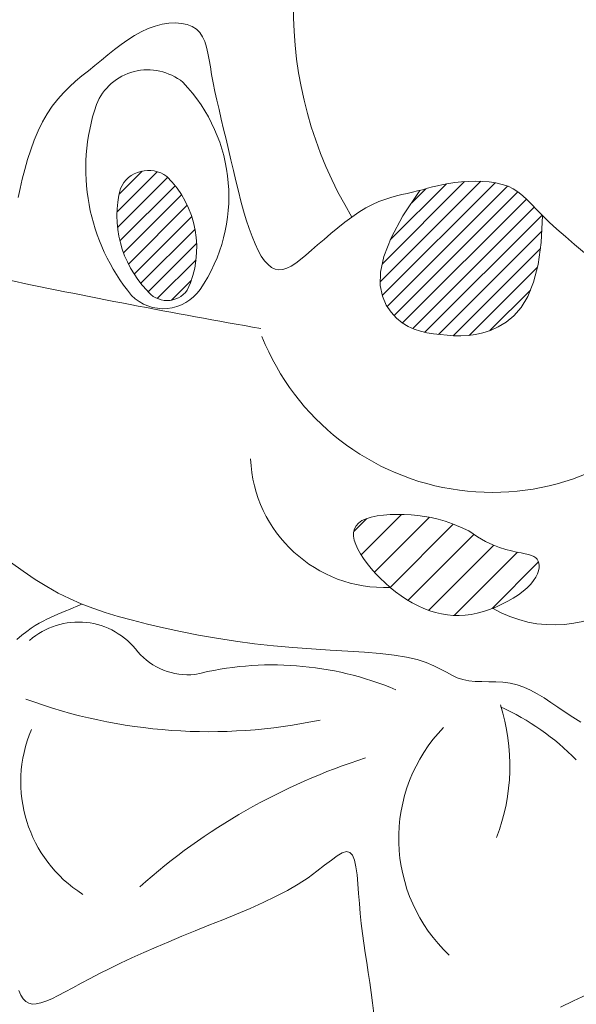
# Model space of a CAD drawing. Units: inches. Extents: x -17 to 1735, y -531 to 60.
# Tile 8 of 27: x 1734.673629 to 1734.675388, y -150.221388 to -150.218274. Entities that reach past the tile are written whole.
import ezdxf

# ---------------------------------------------------------------- set-up
doc = ezdxf.new("R2010")
doc.units = ezdxf.units.IN
doc.header["$MEASUREMENT"] = 0
doc.layers.add('A-FURN', color=242, linetype='Continuous', lineweight=18, true_color=0xcd2027)

# ---------------------------------------------------------------- blocks, each defined once
blk = doc.blocks.new('childrens_room_2')
for p, q in [((70.1409893039486, 54.10887213346581), (70.14043128957158, 54.10867226080739)), ((70.1415457864164, 54.10901436526041), (70.1409893039486, 54.10887213346581)), ((70.14209103538772, 54.10909844610291), (70.1415457864164, 54.10901436526041)), ((70.14261534933351, 54.10912386588319), (70.14209103538772, 54.10909844610291)), ((70.14310902649189, 54.10909011452026), (70.14261534933351, 54.10912386588319)), ((70.14356236527559, 54.10899668191126), (70.14310902649189, 54.10909011452026)), ((70.14396566403914, 54.10884305795338), (70.14356236527559, 54.10899668191126)), ((70.1443092211953, 54.10862873255831), (70.14396566403914, 54.10884305795338)), ((70.13933517482249, 54.10811183522895), (70.1387968190352, 54.1077663301316)), ((70.13987965789741, 54.10841653263054), (70.13933517482249, 54.10811183522895)), ((70.14043128957158, 54.10867226080739), (70.13987965789741, 54.10841653263054)), ((70.14458682429861, 54.10835379073836), (70.1443092211953, 54.10862873255831)), ((70.14480621752912, 54.10802069795903), (70.14458682429861, 54.10835379073836)), ((70.14497863449972, 54.10763251480097), (70.14480621752912, 54.10802069795903)), ((70.13826356939856, 54.10738817888199), (70.13773440460093, 54.10698554301638)), ((70.1387968190352, 54.1077663301316), (70.13826356939856, 54.10738817888199)), ((70.14511530859048, 54.10719230183753), (70.14497863449972, 54.10763251480097)), ((70.14522747323964, 54.10670311964935), (70.14511530859048, 54.10719230183753)), ((70.13720830350533, 54.106566584071), (70.13668424485834, 54.10613946358211)), ((70.13773440460093, 54.10698554301638), (70.13720830350533, 54.106566584071)), ((70.14532636200195, 54.10616802881708), (70.14522747323964, 54.10670311964935)), ((70.13616120746477, 54.10571234308594), (70.13563902106719, 54.1052905785968)), ((70.13668424485834, 54.10613946358211), (70.13616120746477, 54.10571234308594)), ((70.14542320831563, 54.10559008991407), (70.14532636200195, 54.10616802881708)), ((70.14552924561897, 54.10497236352097), (70.14542320831563, 54.10559008991407)), ((70.13512091956684, 54.10486830399753), (70.13461098786095, 54.10443684767819)), ((70.13563902106719, 54.1052905785968), (70.13512091956684, 54.10486830399753)), ((70.14565340960283, 54.10431791021841), (70.14552924561897, 54.10497236352097)), ((70.13411331084674, 54.10398753798512), (70.13363197342144, 54.10351170330108)), ((70.13461098786095, 54.10443684767819), (70.13411331084674, 54.10398753798512)), ((70.14579544502661, 54.10362979057248), (70.14565340960283, 54.10431791021841)), ((70.13363197342144, 54.10351170330108), (70.13317106054049, 54.10300067199426)), ((70.14595279878588, 54.10291106516382), (70.14579544502661, 54.10362979057248)), ((70.1327346569847, 54.1024457724256), (70.1323268477677, 54.10183833297054)), ((70.13317106054049, 54.10300067199426), (70.1327346569847, 54.1024457724256)), ((70.14612291789265, 54.10216479456579), (70.14595279878588, 54.10291106516382)), ((70.1323268477677, 54.10183833297054), (70.13195086667432, 54.10117316764666)), ((70.14630324918429, 54.10139403935176), (70.14612291789265, 54.10216479456579)), ((70.13195086667432, 54.10117316764666), (70.13160654356354, 54.1004590331126)), ((70.14649123967277, 54.10060186009508), (70.14630324918429, 54.10139403935176)), ((70.13160654356354, 54.1004590331126), (70.13129285718199, 54.09970817165453)), ((70.14668433631189, 54.09979131736912), (70.14649123967277, 54.10060186009508)), ((70.13129285718199, 54.09970817165453), (70.13100878633443, 54.09893282558044)), ((70.14687998593902, 54.09896547175453), (70.14668433631189, 54.09979131736912)), ((70.13100878633443, 54.09893282558044), (70.13075330982568, 54.09814523720564)), ((70.14707623132156, 54.09812823396936), (70.14687998593902, 54.09896547175453)), ((70.13075330982568, 54.09814523720564), (70.1305254063441, 54.09735764880901)), ((70.14727349795751, 54.09728691541244), (70.14707623132156, 54.09812823396936)), ((70.1305254063441, 54.09735764880901), (70.1303240547527, 54.09658230270583)), ((70.13792845654417, 54.09393505760675), (70.14116838924704, 54.09717499032416)), ((70.13809711784009, 54.09537651111026), (70.13995124435635, 54.09723063762652)), ((70.14747280698387, 54.09644967761273), (70.14727349795751, 54.09728691541244)), ((70.1303240547527, 54.09658230270583), (70.1301482338563, 54.09583144119682)), ((70.13797547931202, 54.09270928815243), (70.14199178125592, 54.09672559012546)), ((70.13816464070581, 54.09162565735318), (70.14259264316527, 54.09605365979809)), ((70.14767517977046, 54.09562468211373), (70.14747280698387, 54.09644967761273)), ((70.15907037753962, 54.08834834226439), (70.16712777678507, 54.09640574153167)), ((70.1592271576624, 54.0872323302014), (70.16828360648243, 54.09628877902145)), ((70.15923180711573, 54.08978256406266), (70.16583344911808, 54.09638420604318)), ((70.15987140628161, 54.09169495545069), (70.16437979241485, 54.09620334157665)), ((70.16366790474743, 54.09605469296224), (70.16325226613438, 54.09595114353436)), ((70.164101925398, 54.096151101045), (70.16366790474743, 54.09605469296224)), ((70.16456045543192, 54.09623730720927), (70.164101925398, 54.096151101045)), ((70.16504962225329, 54.09631025088896), (70.16456045543192, 54.09623730720927)), ((70.16557265970508, 54.09636678649116), (70.16504962225329, 54.09631025088896)), ((70.16612122779362, 54.09640342835195), (70.16557265970508, 54.09636678649116)), ((70.16668409296427, 54.09641660580968), (70.16612122779362, 54.09640342835195)), ((70.16725002189517, 54.0964027481736), (70.16668409296427, 54.09641660580968)), ((70.16780778097339, 54.09635828478934), (70.16725002189517, 54.0964027481736)), ((70.16834613681888, 54.09627964495888), (70.16780778097339, 54.09635828478934)), ((70.16885385587696, 54.09616325802057), (70.16834613681888, 54.09627964495888)), ((70.16931970470935, 54.09600555330547), (70.16885385587696, 54.09616325802057)), ((70.1301482338563, 54.09583144119682), (70.12999662443647, 54.09511539372619)), ((70.1384615440725, 54.09064976854137), (70.14312020183891, 54.09530842628595)), ((70.14788163739607, 54.09482009045899), (70.14767517977046, 54.09562468211373)), ((70.15962358274149, 54.08635596305106), (70.16928494146444, 54.09601732177401)), ((70.16017334769597, 54.08563293579795), (70.17010568234721, 54.09556527044191)), ((70.16080813407783, 54.09533562778818), (70.16036577337539, 54.09523063297678)), ((70.16123619758174, 54.0954314408504), (70.16080813407783, 54.09533562778818)), ((70.16088463407824, 54.09363122643703), (70.16225299740793, 54.09568155790333)), ((70.16165098525701, 54.09552674379523), (70.16123619758174, 54.0954314408504)), ((70.16158640251845, 54.09468274388058), (70.16270888149623, 54.09580522286564)), ((70.16205436912017, 54.0956282528918), (70.16165098525701, 54.09552674379523)), ((70.1624516256957, 54.09573486292214), (70.16205436912017, 54.0956282528918)), ((70.16284888227122, 54.09584351332745), (70.1624516256957, 54.09573486292214)), ((70.16325226613438, 54.09595114353436), (70.16284888227122, 54.09584351332745)), ((70.1697372155136, 54.09580355523798), (70.16931970470935, 54.09600555330547)), ((70.17011898343802, 54.09555666871023), (70.1697372155136, 54.09580355523798)), ((70.1704823693249, 54.09526489372223), (70.17011898343802, 54.09555666871023)), ((70.17084473395838, 54.09492823028125), (70.1704823693249, 54.09526489372223)), ((70.13884727908183, 54.08976271130672), (70.14356995939627, 54.09448539164299)), ((70.14809320123052, 54.09404406418474), (70.14788163739607, 54.09482009045899)), ((70.15843293467654, 54.09454540371228), (70.15790376987891, 54.09426442574335)), ((70.15894269618323, 54.09477384179485), (70.15843293467654, 54.09454540371228)), ((70.1594340756524, 54.09495841160827), (70.15894269618323, 54.09477384179485)), ((70.15990809433745, 54.09510778479893), (70.1594340756524, 54.09495841160827)), ((70.16036577337539, 54.09523063297678), (70.15990809433745, 54.09510778479893)), ((70.16084164999077, 54.08502844591424), (70.17079118512223, 54.09497798106753)), ((70.17122343823895, 54.09454667837275), (70.17084473395838, 54.09492823028125)), ((70.17163584289258, 54.09412023801127), (70.17122343823895, 54.09454667837275)), ((70.14831089235261, 54.09330476484178), (70.14809320123052, 54.09404406418474)), ((70.15735554230515, 54.09392572190558), (70.15679403878633, 54.09353804885762)), ((70.15790376987891, 54.09426442574335), (70.15735554230515, 54.09392572190558)), ((70.1616657237278, 54.08457972743639), (70.17142463272786, 54.09433863645102)), ((70.1626409005362, 54.08428211201538), (70.17205388856704, 54.09369510007531)), ((70.17209930887796, 54.09364890918226), (70.17163584289258, 54.09412023801127)), ((70.1393106744031, 54.08895331444949), (70.14393328998588, 54.09357593001772)), ((70.14853573207395, 54.09261035395906), (70.14831089235261, 54.09330476484178)), ((70.15622640797984, 54.09311364889294), (70.15565979836859, 54.09266476431952)), ((70.15679403878633, 54.09353804885762), (70.15622640797984, 54.09311364889294)), ((70.1599383932294, 54.09186810651448), (70.16088463407824, 54.09363122643703)), ((70.17209930887796, 54.09364890918226), (70.1719896525133, 54.09150446250572)), ((70.17263119697921, 54.09313269190755), (70.17209930887796, 54.09364890918226)), ((70.17324350653101, 54.09257243632459), (70.17263119697921, 54.09313269190755)), ((70.13984510513139, 54.08821495293381), (70.14419506136213, 54.09256490920819)), ((70.14876857144876, 54.09196839797226), (70.14853573207395, 54.09261035395906)), ((70.15510135855178, 54.09220363744537), (70.15455823712867, 54.09174251057123)), ((70.15565979836859, 54.09266476431952), (70.15510135855178, 54.09220363744537)), ((70.16374023003621, 54.08410864933689), (70.17203565414414, 54.09240407345208)), ((70.1739267913031, 54.09197239324424), (70.17324350653101, 54.09257243632459)), ((70.14043469169295, 54.08753174733141), (70.14432797663497, 54.09142503227343)), ((70.14900958061801, 54.09138408285656), (70.14876857144876, 54.09196839797226)), ((70.14925875963993, 54.09086199947927), (70.14900958061801, 54.09138408285656)), ((70.15403758264031, 54.09129362599782), (70.15354654368596, 54.09086922604041)), ((70.15455823712867, 54.09174251057123), (70.15403758264031, 54.09129362599782)), ((70.1593574794347, 54.0903665324426), (70.1599383932294, 54.09186810651448)), ((70.1719896525133, 54.09150446250572), (70.17173998460524, 54.08973568610822)), ((70.17466624338297, 54.09133766362941), (70.1739267913031, 54.09197239324424)), ((70.17544705514914, 54.09067334845025), (70.17466624338297, 54.09133766362941)), ((70.1495161083981, 54.09040673870044), (70.14925875963993, 54.09086199947927)), ((70.15354654368596, 54.09086922604041), (70.15309048165685, 54.09048061781362)), ((70.16490909830785, 54.08400472543002), (70.1719207591482, 54.09101638622672)), ((70.14116719552433, 54.08699145893336), (70.14427654911881, 54.09010081250603)), ((70.14978162700893, 54.0900228913801), (70.1495161083981, 54.09040673870044)), ((70.15005531541422, 54.08971504838558), (70.14978162700893, 54.0900228913801)), ((70.15033717361396, 54.08948780058421), (70.15005531541422, 54.08971504838558)), ((70.15227435268346, 54.08984010710122), (70.15190713713994, 54.08960146711473)), ((70.15266760940315, 54.09013536774586), (70.15227435268346, 54.08984010710122)), ((70.15309048165685, 54.09048061781362), (70.15266760940315, 54.09013536774586)), ((70.15908509709291, 54.08910083852828), (70.1593574794347, 54.0903665324426)), ((70.17173998460524, 54.08973568610822), (70.17137219559984, 54.08830158180939)), ((70.15062720160816, 54.08934573883602), (70.15033717361396, 54.08948780058421)), ((70.15092599509401, 54.08929158365066), (70.15062720160816, 54.08934573883602)), ((70.15123653267393, 54.08932057414353), (70.15092599509401, 54.08929158365066)), ((70.15156238858938, 54.08942607904322), (70.15123653267393, 54.08932057414353)), ((70.15190713713994, 54.08960146711473), (70.15156238858938, 54.08942607904322)), ((70.1590644508938, 54.08804535909297), (70.15908509709291, 54.08910083852828)), ((70.16620839743294, 54.08403123232568), (70.17168036016986, 54.08950319506988)), ((70.14231109433925, 54.08686256552613), (70.14389058733244, 54.08844205856297)), ((70.17137219559984, 54.08830158180939), (70.1709081759432, 54.08716115143619)), ((70.15923874523608, 54.0871744284363), (70.1590644508938, 54.08804535909297)), ((70.16787284421619, 54.08442288687223), (70.17111196486395, 54.08766200757094)), ((70.15955118469313, 54.08646238087243), (70.15923874523608, 54.0871744284363)), ((70.1709081759432, 54.08716115143619), (70.17036981608138, 54.08627339679373)), ((70.15994497378009, 54.08588355070827), (70.15955118469313, 54.08646238087243)), ((70.16037242878113, 54.08541446645398), (70.15994497378009, 54.08588355070827)), ((70.17036981608138, 54.08627339679373), (70.16977900640225, 54.08559731971621)), ((70.16082231311478, 54.08504043337456), (70.16037242878113, 54.08541446645398)), ((70.16129250179395, 54.08474895096009), (70.16082231311478, 54.08504043337456)), ((70.1691576372937, 54.08509192200148), (70.1685275993182, 54.08471620548374)), ((70.16977900640225, 54.08559731971621), (70.1691576372937, 54.08509192200148)), ((70.1617808700062, 54.08452751865701), (70.16129250179395, 54.08474895096009)), ((70.16228529288085, 54.08436363595541), (70.1617808700062, 54.08452751865701)), ((70.16280364548903, 54.08424480231627), (70.16228529288085, 54.08436363595541)), ((70.16333380296012, 54.08415851721514), (70.16280364548903, 54.08424480231627)), ((70.16729894659832, 54.08423096492919), (70.16670268169722, 54.08409601430907)), ((70.1679070163623, 54.08443431467316), (70.16729894659832, 54.08423096492919)), ((70.1685275993182, 54.08471620548374), (70.1679070163623, 54.08443431467316)), ((70.16387364048163, 54.084092280113), (70.16333380296012, 54.08415851721514)), ((70.16442150530521, 54.08403736424083), (70.16387364048163, 54.084092280113)), ((70.1649776335212, 54.08400013777868), (70.16442150530521, 54.08403736424083)), ((70.16554273351679, 54.0839907426693), (70.1649776335212, 54.08400013777868)), ((70.16611751344638, 54.08401932087002), (70.16554273351679, 54.0839907426693)), ((70.16670268169722, 54.08409601430907), (70.16611751344638, 54.08401932087002)), ((70.15694353497705, 54.06828989399077), (70.15797352163239, 54.06931988068248)), ((70.15731488378836, 54.06896104964693), (70.15758673929261, 54.06915109147525)), ((70.15752426960854, 54.06640090262084), (70.16076704901528, 54.069643682013)), ((70.15758673929261, 54.06915109147525), (70.15793346800959, 54.06930778243844)), ((70.15793346800959, 54.06930778243844), (70.15834586818121, 54.06943234820068)), ((70.15834586818121, 54.06943234820068), (70.15881212289563, 54.06952672402116)), ((70.15859754279839, 54.06500444983834), (70.1630163224286, 54.06942322947583)), ((70.15881212289563, 54.06952672402116), (70.15932041512454, 54.06959284515181)), ((70.15932041512454, 54.06959284515181), (70.15985892789789, 54.06963264684458)), ((70.15985892789789, 54.06963264684458), (70.16041584418738, 54.06964806436594)), ((70.16041584418738, 54.06964806436594), (70.16097934708117, 54.06964103295326)), ((70.16097934708117, 54.06964103295326), (70.16153761943454, 54.06961348786575)), ((70.16153761943454, 54.06961348786575), (70.16208233144019, 54.06956626772302)), ((70.16208233144019, 54.06956626772302), (70.16261910083588, 54.06949582454257)), ((70.16261910083588, 54.06949582454257), (70.16315703252215, 54.06939751371687)), ((70.16315703252215, 54.06939751371687), (70.16370523145773, 54.06926669061653)), ((70.16370523145773, 54.06926669061653), (70.16427280242672, 54.06909871063402)), ((70.15692550416455, 54.06820978447507), (70.15698814067176, 54.06848807385398)), ((70.15698814067176, 54.06848807385398), (70.15711664246513, 54.06873926967676)), ((70.15711664246513, 54.06873926967676), (70.15731488378836, 54.06896104964693)), ((70.15985669091927, 54.06379387196506), (70.16492787831115, 54.06886505934966)), ((70.16427280242672, 54.06909871063402), (70.16486885027146, 54.06888892915453)), ((70.16486885027146, 54.06888892915453), (70.16550247995067, 54.06863270154866)), ((70.16550247995067, 54.06863270154866), (70.16618279630669, 54.06832538321618)), ((70.15692485846697, 54.06790672385835), (70.15692550416455, 54.06820978447507)), ((70.15698232910248, 54.06758121430033), (70.15692485846697, 54.06790672385835)), ((70.15709404165275, 54.06723557809749), (70.15698232910248, 54.06758121430033)), ((70.16129145702465, 54.06275891204717), (70.16658396752203, 54.06805142253)), ((70.16618279630669, 54.06832538321618), (70.16686627735501, 54.06785863249973)), ((70.16686627735501, 54.06785863249973), (70.16750345904032, 54.06748961203851)), ((70.15725612175768, 54.06687213756089), (70.15709404165275, 54.06723557809749)), ((70.15746463044663, 54.06649356977727), (70.15725612175768, 54.06687213756089)), ((70.16295105697237, 54.06194878599348), (70.16817510856664, 54.06717283760958)), ((70.16750345904032, 54.06748961203851), (70.16809453501949, 54.06720458154308)), ((70.16809453501949, 54.06720458154308), (70.16863969906584, 54.06698980071673)), ((70.16863969906584, 54.06698980071673), (70.16913914489444, 54.06683152927001)), ((70.16913914489444, 54.06683152927001), (70.16959306616221, 54.06671602689897)), ((70.15771537030699, 54.06610397104526), (70.15746463044663, 54.06649356977727)), ((70.15800407949021, 54.06570779243924), (70.15771537030699, 54.06610397104526)), ((70.16500926205075, 54.06153726508495), (70.1700851896999, 54.06661319274866)), ((70.16959306616221, 54.06671602689897), (70.17000165670063, 54.06662955331416)), ((70.17000165670063, 54.06662955331416), (70.17036511016661, 54.06655836822614)), ((70.17036511016661, 54.06655836822614), (70.17068387854263, 54.06649040855558)), ((70.17068387854263, 54.06649040855558), (70.17095944711357, 54.06642032009989)), ((70.17095944711357, 54.06642032009989), (70.1711935593153, 54.06634442588842)), ((70.1711935593153, 54.06634442588842), (70.17138795870008, 54.06625904893593)), ((70.17138795870008, 54.06625904893593), (70.17154438864557, 54.06616051225722)), ((70.17154438864557, 54.06616051225722), (70.17166459270405, 54.06604513887436)), ((70.17166459270405, 54.06604513887436), (70.17175031442778, 54.06590925180939)), ((70.12938824494952, 54.06582249374918), (70.13038629923133, 54.06508380538292)), ((70.15832649626421, 54.06530948504808), (70.15800407949021, 54.06570779243924)), ((70.15867835860584, 54.06491349994616), (70.15832649626421, 54.06530948504808)), ((70.1680364764866, 54.06209475351937), (70.17177534610849, 54.06583362314126)), ((70.17175031442778, 54.06590925180939), (70.17180329719443, 54.06574917408438)), ((70.17181182089146, 54.06535128597756), (70.17176232505474, 54.06511924909722)), ((70.17180329719443, 54.06574917408438), (70.17182450963767, 54.06556242212395)), ((70.17182450963767, 54.06556242212395), (70.17181182089146, 54.06535128597756)), ((70.13038629923133, 54.06508380538292), (70.13135836332688, 54.06442877838566)), ((70.13135836332688, 54.06442877838566), (70.13229673647905, 54.06385020058809)), ((70.1590554047248, 54.06452428822234), (70.15867835860584, 54.06491349994616)), ((70.15945337271435, 54.06414630095827), (70.1590554047248, 54.06452428822234)), ((70.17154128902942, 54.06460640696463), (70.17136393715512, 54.06433256862368)), ((70.17167311640108, 54.06486979494224), (70.17154128902942, 54.06460640696463)), ((70.17176232505474, 54.06511924909722), (70.17167311640108, 54.06486979494224)), ((70.13229673647905, 54.06385020058809), (70.13321296988173, 54.06333893653794)), ((70.15986800066779, 54.06378398922829), (70.15945337271435, 54.06414630095827)), ((70.16029547889369, 54.06344138482968), (70.15986800066779, 54.06378398922829)), ((70.17086103670184, 54.06376747465987), (70.17053141993122, 54.06348331496559)), ((70.17113815499354, 54.06405176337142), (70.17086103670184, 54.06376747465987)), ((70.17136393715512, 54.06433256862368), (70.17113815499354, 54.06405176337142)), ((70.13321296988173, 54.06333893653794), (70.13412342757104, 54.06288536999494)), ((70.13412342757104, 54.06288536999494), (70.13504447393237, 54.06247988471881)), ((70.16073380545598, 54.0631208422987), (70.16029547889369, 54.06344138482968)), ((70.16118143063389, 54.0628242969164), (70.16073380545598, 54.0631208422987)), ((70.16163680464845, 54.06255368392016), (70.16118143063389, 54.0628242969164)), ((70.16973968119012, 54.06293202581441), (70.16929266934633, 54.06267341146161)), ((70.1701551164256, 54.06320341283429), (70.16973968119012, 54.06293202581441)), ((70.17053141993122, 54.06348331496559), (70.1701551164256, 54.06320341283429)), ((70.13381352038007, 54.06189630216835), (70.13412075077534, 54.06202414168223)), ((70.13412075077534, 54.06202414168223), (70.13440788049368, 54.06214337407295)), ((70.13440788049368, 54.06214337407295), (70.13466391713476, 54.06224951902408)), ((70.13466391713476, 54.06224951902408), (70.13487786853104, 54.06233809618282)), ((70.13487786853104, 54.06233809618282), (70.13503874234041, 54.06240462523277)), ((70.13503874234041, 54.06240462523277), (70.1351355462789, 54.06244462582112)), ((70.13504447393237, 54.06247988471881), (70.13599247300183, 54.06211286444744)), ((70.13599247300183, 54.06211286444744), (70.1369837890484, 54.06177469293329)), ((70.1620983777789, 54.06231093857645), (70.16163680464845, 54.06255368392016)), ((70.16256460024627, 54.06209799614448), (70.1620983777789, 54.06231093857645)), ((70.16303392227158, 54.06191679187617), (70.16256460024627, 54.06209799614448)), ((70.16833413655289, 54.06221153099472), (70.16783772578813, 54.06201677999201)), ((70.168821636074, 54.06243182733163), (70.16833413655289, 54.06221153099472)), ((70.16929266934633, 54.06267341146161), (70.168821636074, 54.06243182733163)), ((70.13199226559257, 54.06108987538613), (70.1322883098724, 54.06123859779331)), ((70.1322883098724, 54.06123859779331), (70.13258202177124, 54.06137478726162)), ((70.13258202177124, 54.06137478726162), (70.13287847088534, 54.06150423272487)), ((70.13287847088534, 54.06150423272487), (70.1331827266363, 54.06163272313136)), ((70.1331827266363, 54.06163272313136), (70.13349718159182, 54.06176433587683)), ((70.13349718159182, 54.06176433587683), (70.13381352038007, 54.06189630216835)), ((70.1369837890484, 54.06177469293329), (70.13803478622461, 54.06145575393606)), ((70.13803478622461, 54.06145575393606), (70.13916182874121, 54.06114643120822)), ((70.16350479407586, 54.06176926102347), (70.16303392227158, 54.06191679187617)), ((70.16397605336854, 54.06165698405533), (70.16350479407586, 54.06176926102347)), ((70.1644480875216, 54.06158012223608), (70.16397605336854, 54.06165698405533)), ((70.16492167151183, 54.06153848203979), (70.1644480875216, 54.06158012223608)), ((70.16539758014144, 54.06153186993328), (70.16492167151183, 54.06153848203979)), ((70.16587658832898, 54.06156009239061), (70.16539758014144, 54.06153186993328)), ((70.16635947093485, 54.06162295589314), (70.16587658832898, 54.06156009239061)), ((70.16684700287763, 54.06172026690041), (70.16635947093485, 54.06162295589314)), ((70.1673399589595, 54.06185183188648), (70.16684700287763, 54.06172026690041)), ((70.16783772578813, 54.06201677999201), (70.1673399589595, 54.06185183188648)), ((70.13068337576581, 54.0602538774678), (70.13103944413481, 54.0605106210773)), ((70.13103944413481, 54.0605106210773), (70.1313729022618, 54.06073167596918)), ((70.1313729022618, 54.06073167596918), (70.13168881956838, 54.06092283109177)), ((70.13168881956838, 54.06092283109177), (70.13199226559257, 54.06108987538613)), ((70.13916182874121, 54.06114643120822), (70.14037662821241, 54.06083951255863)), ((70.14037662821241, 54.06083951255863), (70.14167228598265, 54.06053740204374)), ((70.14167228598265, 54.06053740204374), (70.14303725091625, 54.06024490779822)), ((70.12990142278025, 54.05961865505236), (70.13030191418832, 54.0599567170488)), ((70.13030191418832, 54.0599567170488), (70.13068337576581, 54.0602538774678)), ((70.14303725091625, 54.06024490779822), (70.1444599717611, 54.05996683792768)), ((70.1444599717611, 54.05996683792768), (70.14592889732333, 54.05970800055951)), ((70.14592889732333, 54.05970800055951), (70.14743247646723, 54.05947320382842)), ((70.14743247646723, 54.05947320382842), (70.1489591579407, 54.05926725583999)), ((70.1489591579407, 54.05926725583999), (70.15049739060808, 54.05909496472162)), ((70.15049739060808, 54.05909496472162), (70.15203433979653, 54.05895857426952)), ((70.15203433979653, 54.05895857426952), (70.15355203697575, 54.05885007092587)), ((70.15355203697575, 54.05885007092587), (70.15503123013653, 54.05875887683072)), ((70.15503123013653, 54.05875887683072), (70.15645266744426, 54.05867441410231)), ((70.15645266744426, 54.05867441410231), (70.1577970967733, 54.05858610486615)), ((70.1577970967733, 54.05858610486615), (70.15904526628904, 54.05848337124047)), ((70.15904526628904, 54.05848337124047), (70.16017792398227, 54.05835563535077)), ((70.16017792398227, 54.05835563535077), (70.16117581784377, 54.05819231932986)), ((70.16117581784377, 54.05819231932986), (70.1620269154769, 54.05798685207122)), ((70.1620269154769, 54.05798685207122), (70.16274806223694, 54.05774868954762)), ((70.16274806223694, 54.05774868954762), (70.16336332320817, 54.05749129452164)), ((70.16336332320817, 54.05749129452164), (70.1638967632421, 54.0572281297413)), ((70.1638967632421, 54.0572281297413), (70.16437244742295, 54.0569726579692)), ((70.16437244742295, 54.0569726579692), (70.164814440544, 54.05673834194607)), ((70.164814440544, 54.05673834194607), (70.16524680774776, 54.05653864443451)), ((70.16524680774776, 54.05653864443451), (70.16569361388568, 54.05638702818254)), ((70.16569361388568, 54.05638702818254), (70.16617379006814, 54.05629198755781)), ((70.16617379006814, 54.05629198755781), (70.1666857319756, 54.05624214331914)), ((70.1666857319756, 54.05624214331914), (70.16722270148924, 54.05622114783767)), ((70.16722270148924, 54.05622114783767), (70.16777796031559, 54.05621265349186)), ((70.16777796031559, 54.05621265349186), (70.16834477033584, 54.0562003126601)), ((70.16834477033584, 54.0562003126601), (70.16891639337294, 54.05616777770632)), ((70.16891639337294, 54.05616777770632), (70.16948609124987, 54.05609870100164)), ((70.16948609124987, 54.05609870100164), (70.17004712567316, 54.05597673492451)), ((70.17004712567316, 54.05597673492451), (70.17059491488502, 54.05578987813209)), ((70.17059491488502, 54.05578987813209), (70.17113350216415, 54.05554351444738)), ((70.17113350216415, 54.05554351444738), (70.17166908697575, 54.05524737395757)), ((70.17166908697575, 54.05524737395757), (70.17220786901773, 54.05491118677895)), ((70.17220786901773, 54.05491118677895), (70.17275604781346, 54.05454468300598)), ((70.17275604781346, 54.05454468300598), (70.17331982294446, 54.05415759274768)), ((70.17331982294446, 54.05415759274768), (70.17390539405054, 54.05375964609124)), ((70.17390539405054, 54.05375964609124), (70.17451896065498, 54.0533605731602)), ((70.17451896065498, 54.0533605731602), (70.17516499910155, 54.05296905373546)), ((70.15601189272596, 54.0424676478346), (70.15561111284072, 54.04223452806622)), ((70.15634577990161, 54.04256711738566), (70.15601189272596, 54.0424676478346)), ((70.15661623434747, 54.04250758927668), (70.15634577990161, 54.04256711738566)), ((70.15682777309442, 54.04227216519069), (70.15661623434747, 54.04250758927668)), ((70.15698914230919, 54.04187774344467), (70.15682777309442, 54.04227216519069)), ((70.15459503484774, 54.04146872772111), (70.15397281689685, 54.04098674205164)), ((70.1551399801497, 54.04189310554506), (70.15459503484774, 54.04146872772111)), ((70.15561111284072, 54.04223452806622), (70.1551399801497, 54.04189310554506)), ((70.15711014515139, 54.0413496714886), (70.15698914230919, 54.04187774344467)), ((70.15397281689685, 54.04098674205164), (70.15326986631729, 54.04047249598665)), ((70.15720058495529, 54.04071329677975), (70.15711014515139, 54.0413496714886)), ((70.15727026493872, 54.0399939667754), (70.15720058495529, 54.04071329677975)), ((70.15248272312922, 54.03995133699067), (70.1516108107858, 54.03944400389304)), ((70.15326986631729, 54.04047249598665), (70.15248272312922, 54.03995133699067)), ((70.1573289883195, 54.03921702894007), (70.15727026493872, 54.0399939667754)), ((70.1516108107858, 54.03944400389304), (70.15066508577323, 54.03895280098954)), ((70.1573865583737, 54.03840783073104), (70.1573289883195, 54.03921702894007)), ((70.14965938795243, 54.03847542398438), (70.14860755724251, 54.0380095685527)), ((70.15066508577323, 54.03895280098954), (70.14965938795243, 54.03847542398438)), ((70.15745277831914, 54.03759171959831), (70.1573865583737, 54.03840783073104)), ((70.1475234334462, 54.03755293038415), (70.14642085648259, 54.03710320516115)), ((70.14860755724251, 54.0380095685527), (70.1475234334462, 54.03755293038415)), ((70.15753524093773, 54.03678895431079), (70.15745277831914, 54.03759171959831)), ((70.14642085648259, 54.03710320516115), (70.1453136661544, 54.0366580885588)), ((70.15763269680204, 54.0359994388404), (70.15753524093773, 54.03678895431079)), ((70.14421570243897, 54.03621527628132), (70.1431390751491, 54.0357730400778)), ((70.1453136661544, 54.0366580885588), (70.14421570243897, 54.03621527628132)), ((70.15774168581586, 54.03521798849254), (70.15763269680204, 54.0359994388404)), ((70.14208897425445, 54.03533195603671), (70.14106885973482, 54.03489317630596)), ((70.1431390751491, 54.0357730400778), (70.14208897425445, 54.03533195603671)), ((70.15785874817405, 54.03443941855079), (70.15774168581586, 54.03521798849254)), ((70.14008219156997, 54.03445785304796), (70.1391324297397, 54.03402713842519)), ((70.14106885973482, 54.03489317630596), (70.14008219156997, 54.03445785304796)), ((70.1579804237804, 54.03365854430598), (70.15785874817405, 54.03443941855079)), ((70.13822303422378, 54.0336021845855), (70.13735746494379, 54.03318414369135)), ((70.1391324297397, 54.03402713842519), (70.13822303422378, 54.0336021845855)), ((70.15810325271335, 54.03287018103441), (70.1579804237804, 54.03365854430598)), ((70.13653918199591, 54.03277416790519), (70.13577106858023, 54.03237436950298)), ((70.13735746494379, 54.03318414369135), (70.13653918199591, 54.03277416790519)), ((70.1582237749931, 54.03206914404148), (70.15810325271335, 54.03287018103441)), ((70.13505370141823, 54.03199070130217), (70.13438708050992, 54.03163007624101)), ((70.13577106858023, 54.03237436950298), (70.13505370141823, 54.03199070130217)), ((70.1583385306981, 54.0312502486035), (70.1582237749931, 54.03206914404148)), ((70.13021666388843, 54.03103671543653), (70.13004914369552, 54.03141865540096)), ((70.13377120585531, 54.03129940725779), (70.13320607739618, 54.03100560729075)), ((70.13438708050992, 54.03163007624101), (70.13377120585531, 54.03129940725779)), ((70.15844540531864, 54.03041195851841), (70.1583385306981, 54.0312502486035)), ((70.13040379051702, 54.03074003508521), (70.13021666388843, 54.03103671543653)), ((70.13061571360916, 54.0305251578597), (70.13040379051702, 54.03074003508521)), ((70.13085762307631, 54.03038862730176), (70.13061571360916, 54.0305251578597)), ((70.13181516959915, 54.03041455086935), (70.13145216113072, 54.03033678027572)), ((70.1322280592972, 54.03055626615827), (70.13181516959915, 54.03041455086935)), ((70.13269169524895, 54.03075558927816), (70.1322280592972, 54.03055626615827)), ((70.13320607739618, 54.03100560729075), (70.13269169524895, 54.03075558927816)), ((70.15854766663281, 54.02956733155446), (70.15844540531864, 54.03041195851841)), ((70.17456501944574, 54.03058353331147), (70.17352318415536, 54.03007965674482)), ((70.17560685473612, 54.03107358400887), (70.17456501944574, 54.03058353331147)), ((70.13113470894633, 54.03032698693135), (70.13085762307631, 54.03038862730176)), ((70.13145216113072, 54.03033678027572), (70.13113470894633, 54.03032698693135))]:
    blk.add_line(p, q)
for centre, radius, start, end in [((70.18419688196039, 54.11024985505941), 0.0320967331381597, 82.95662561159509, 211.3772048657365), ((70.14041021682672, 54.10090234786043), 0.0044570508413919, 50.82799451834666, 158.0159715734295), ((70.1336740135553, 54.09519485259664), 0.0132358904717108, 325.6481931397273, 43.81023854096406), ((70.15139647970094, 54.0974310095466), 0.0159690027647587, 161.2243872807157, 219.6319536606606), ((70.14045053960174, 54.09481264951904), 0.0024690002498248, 53.52143240935108, 155.519311169789), ((70.13634555374622, 54.09107193013046), 0.0079902288067912, 334.7018353736999, 45.77646759189611), ((70.14658124722656, 54.09365320773798), 0.0086573798592064, 165.3979344622773, 223.8328993580882), ((70.25073743193526, 54.66704331015939), 0.5911939097029936, 258.0690127884769, 260.1371981708295), ((70.1416509663791, 54.08975829707054), 0.0035825332570705, 224.548065895743, 325.4431602022488), ((70.1419528130314, 54.08882326674796), 0.0019931670171244, 215.7955336360922, 324.2044663639078), ((70.16805124132544, 54.09132497389368), 0.0199068323432125, 201.8074763810449, 322.9514703004661), ((70.15944396938315, 54.07457986113735), 0.0108041960763789, 182.4908581835723, 272.2492601854808), ((70.17302459694795, 54.07056868865623), 0.0097912997460796, 239.7089148198155, 310.1368033599684), ((70.13483657112695, 54.05505638739708), 0.005950330072877, 36.78744036339995, 131.2066142042287), ((70.14365037671406, 54.06211785731142), 0.0053503736530777, 220.8294581309691, 275.6077019872809), ((70.15041969927145, 54.031920978507), 0.0256445056373721, 67.27867680351453, 104.0979619409809), ((70.14532335074503, 54.09491666771504), 0.0427157227761538, 249.8545836920238, 282.0349049426248), ((70.1533879849699, 54.0494635890413), 0.0160803001751278, 339.0046849133215, 17.71882978746521), ((70.1601908126718, 54.03554020717132), 0.0205155212486357, 44.59191164375336, 65.47851642955993), ((70.14090368333157, 54.04817331256203), 0.0106960804239441, 156.8480326701817, 237.6677103668499), ((70.17340135784937, 54.04362390469618), 0.0128535839600232, 136.1351291117474, 226.7319607519272), ((70.17314686860075, 54.00230586594119), 0.0501667886541437, 107.7091370647402, 131.7306854112385)]:
    blk.add_arc(centre, radius, start, end)

msp = doc.modelspace()

# ---------------------------------------------------------------- block references
at = {"layer": 'A-FURN', "xscale": 0.0393700787401575, "yscale": 0.0393700787401575, "zscale": 0.0393700787401575}
msp.add_blockref('childrens_room_2', (1731.912600860487, -152.3485650223338), dxfattribs=at)

doc.saveas('drawing.dxf')
